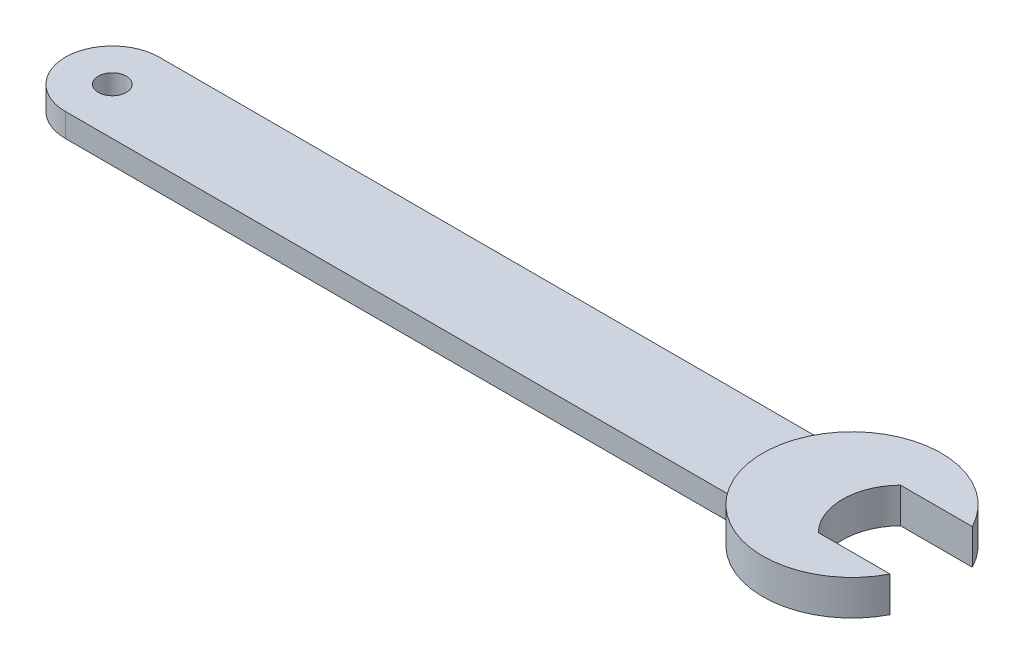
ISO-10303-21;
HEADER;
FILE_DESCRIPTION(('STEP AP214'),'2;1');
FILE_NAME('part.step','',(''),(''),'','','');
FILE_SCHEMA(('AUTOMOTIVE_DESIGN { 1 0 10303 214 1 1 1 1 }'));
ENDSEC;
DATA;
#1=APPLICATION_CONTEXT('core data for automotive mechanical design processes');
#2=APPLICATION_PROTOCOL_DEFINITION('international standard','automotive_design',2000,#1);
#3=PRODUCT_CONTEXT('',#1,'mechanical');
#4=PRODUCT('Part','Part','',(#3));
#5=PRODUCT_RELATED_PRODUCT_CATEGORY('part','',(#4));
#6=PRODUCT_DEFINITION_FORMATION('','',#4);
#7=PRODUCT_DEFINITION_CONTEXT('part definition',#1,'design');
#8=PRODUCT_DEFINITION('design','',#6,#7);
#9=PRODUCT_DEFINITION_SHAPE('','',#8);
#10=(LENGTH_UNIT() NAMED_UNIT(*) SI_UNIT(.MILLI.,.METRE.));
#11=(NAMED_UNIT(*) PLANE_ANGLE_UNIT() SI_UNIT($,.RADIAN.));
#12=(NAMED_UNIT(*) SI_UNIT($,.STERADIAN.) SOLID_ANGLE_UNIT());
#13=UNCERTAINTY_MEASURE_WITH_UNIT(LENGTH_MEASURE(1.E-05),#10,'distance_accuracy_value','');
#14=(GEOMETRIC_REPRESENTATION_CONTEXT(3) GLOBAL_UNCERTAINTY_ASSIGNED_CONTEXT((#13)) GLOBAL_UNIT_ASSIGNED_CONTEXT((#10,
#11,#12)) REPRESENTATION_CONTEXT('',''));
#15=CARTESIAN_POINT('',(0.,0.,0.));
#16=DIRECTION('',(0.,0.,1.));
#17=DIRECTION('',(1.,0.,0.));
#18=AXIS2_PLACEMENT_3D('',#15,#16,#17);
#19=CARTESIAN_POINT('',(0.,5.,-20.));
#20=DIRECTION('',(0.,0.,-1.));
#21=DIRECTION('',(-1.,0.,0.));
#22=AXIS2_PLACEMENT_3D('',#19,#20,#21);
#23=PLANE('',#22);
#24=DIRECTION('',(1.,0.,0.));
#25=VECTOR('',#24,1.);
#26=CARTESIAN_POINT('',(0.,-5.,-20.));
#27=LINE('',#26,#25);
#28=CARTESIAN_POINT('',(-157.5,-5.,-20.));
#29=VERTEX_POINT('',#28);
#30=CARTESIAN_POINT('',(125.189011157193,-5.,-20.0000000000001));
#31=VERTEX_POINT('',#30);
#32=EDGE_CURVE('E100',#29,#31,#27,.T.);
#33=ORIENTED_EDGE('',*,*,#32,.F.);
#34=DIRECTION('',(0.,-1.,0.));
#35=VECTOR('',#34,1.);
#36=CARTESIAN_POINT('',(-157.5,5.,-20.));
#37=LINE('',#36,#35);
#38=CARTESIAN_POINT('',(-157.5,5.,-20.));
#39=VERTEX_POINT('',#38);
#40=EDGE_CURVE('E49',#39,#29,#37,.T.);
#41=ORIENTED_EDGE('',*,*,#40,.F.);
#42=DIRECTION('',(1.,0.,0.));
#43=VECTOR('',#42,1.);
#44=CARTESIAN_POINT('',(0.,5.,-20.));
#45=LINE('',#44,#43);
#46=CARTESIAN_POINT('',(125.189011157193,5.,-20.));
#47=VERTEX_POINT('',#46);
#48=EDGE_CURVE('E111',#39,#47,#45,.T.);
#49=ORIENTED_EDGE('',*,*,#48,.T.);
#50=DIRECTION('',(0.,-1.,0.));
#51=VECTOR('',#50,1.);
#52=CARTESIAN_POINT('',(125.189011157193,5.,-20.0000000000001));
#53=LINE('',#52,#51);
#54=EDGE_CURVE('E11',#47,#31,#53,.T.);
#55=ORIENTED_EDGE('',*,*,#54,.T.);
#56=EDGE_LOOP('',(#33,#41,#49,#55));
#57=FACE_BOUND('',#56,.T.);
#58=ADVANCED_FACE('F41',(#57),#23,.T.);
#59=CARTESIAN_POINT('',(-157.5,5.,0.));
#60=DIRECTION('',(0.,-1.,0.));
#61=DIRECTION('',(0.,0.,-1.));
#62=AXIS2_PLACEMENT_3D('',#59,#60,#61);
#63=CYLINDRICAL_SURFACE('',#62,20.);
#64=CARTESIAN_POINT('',(-157.5,-5.,0.));
#65=DIRECTION('',(0.,1.,0.));
#66=DIRECTION('',(0.,0.,1.));
#67=AXIS2_PLACEMENT_3D('',#64,#65,#66);
#68=CIRCLE('',#67,20.);
#69=CARTESIAN_POINT('',(-157.5,-5.,20.));
#70=VERTEX_POINT('',#69);
#71=EDGE_CURVE('E95',#29,#70,#68,.T.);
#72=ORIENTED_EDGE('',*,*,#71,.T.);
#73=DIRECTION('',(0.,-1.,0.));
#74=VECTOR('',#73,1.);
#75=CARTESIAN_POINT('',(-157.5,5.,20.));
#76=LINE('',#75,#74);
#77=CARTESIAN_POINT('',(-157.5,5.,20.));
#78=VERTEX_POINT('',#77);
#79=EDGE_CURVE('E88',#78,#70,#76,.T.);
#80=ORIENTED_EDGE('',*,*,#79,.F.);
#81=CARTESIAN_POINT('',(-157.5,5.,0.));
#82=DIRECTION('',(0.,1.,0.));
#83=DIRECTION('',(0.,0.,1.));
#84=AXIS2_PLACEMENT_3D('',#81,#82,#83);
#85=CIRCLE('',#84,20.);
#86=EDGE_CURVE('E109',#39,#78,#85,.T.);
#87=ORIENTED_EDGE('',*,*,#86,.F.);
#88=ORIENTED_EDGE('',*,*,#40,.T.);
#89=EDGE_LOOP('',(#72,#80,#87,#88));
#90=FACE_BOUND('',#89,.T.);
#91=ADVANCED_FACE('F108',(#90),#63,.T.);
#92=CARTESIAN_POINT('',(-157.5,5.,0.));
#93=DIRECTION('',(0.,-1.,0.));
#94=DIRECTION('',(0.,0.,-1.));
#95=AXIS2_PLACEMENT_3D('',#92,#93,#94);
#96=CYLINDRICAL_SURFACE('',#95,6.00000000000002);
#97=CARTESIAN_POINT('',(-157.5,5.,0.));
#98=DIRECTION('',(0.,1.,0.));
#99=DIRECTION('',(0.,0.,1.));
#100=AXIS2_PLACEMENT_3D('',#97,#98,#99);
#101=CIRCLE('',#100,6.00000000000002);
#102=CARTESIAN_POINT('',(-157.5,5.,6.00000000000002));
#103=VERTEX_POINT('',#102);
#104=EDGE_CURVE('E93',#103,#103,#101,.T.);
#105=ORIENTED_EDGE('',*,*,#104,.T.);
#106=EDGE_LOOP('',(#105));
#107=FACE_BOUND('',#106,.T.);
#108=CARTESIAN_POINT('',(-157.5,-5.,0.));
#109=DIRECTION('',(0.,1.,0.));
#110=DIRECTION('',(0.,0.,1.));
#111=AXIS2_PLACEMENT_3D('',#108,#109,#110);
#112=CIRCLE('',#111,6.00000000000002);
#113=CARTESIAN_POINT('',(-157.5,-5.,6.00000000000002));
#114=VERTEX_POINT('',#113);
#115=EDGE_CURVE('E98',#114,#114,#112,.T.);
#116=ORIENTED_EDGE('',*,*,#115,.F.);
#117=EDGE_LOOP('',(#116));
#118=FACE_BOUND('',#117,.T.);
#119=ADVANCED_FACE('F43',(#107,#118),#96,.F.);
#120=CARTESIAN_POINT('',(0.,5.,20.));
#121=DIRECTION('',(0.,0.,-1.));
#122=DIRECTION('',(-1.,0.,0.));
#123=AXIS2_PLACEMENT_3D('',#120,#121,#122);
#124=PLANE('',#123);
#125=DIRECTION('',(1.,0.,0.));
#126=VECTOR('',#125,1.);
#127=CARTESIAN_POINT('',(0.,-5.,20.));
#128=LINE('',#127,#126);
#129=CARTESIAN_POINT('',(125.189011157193,-5.,19.9999999999999));
#130=VERTEX_POINT('',#129);
#131=EDGE_CURVE('E71',#70,#130,#128,.T.);
#132=ORIENTED_EDGE('',*,*,#131,.T.);
#133=DIRECTION('',(0.,-1.,0.));
#134=VECTOR('',#133,1.);
#135=CARTESIAN_POINT('',(125.189011157193,5.,19.9999999999999));
#136=LINE('',#135,#134);
#137=CARTESIAN_POINT('',(125.189011157193,5.,20.));
#138=VERTEX_POINT('',#137);
#139=EDGE_CURVE('E79',#138,#130,#136,.T.);
#140=ORIENTED_EDGE('',*,*,#139,.F.);
#141=DIRECTION('',(1.,0.,0.));
#142=VECTOR('',#141,1.);
#143=CARTESIAN_POINT('',(0.,5.,20.));
#144=LINE('',#143,#142);
#145=EDGE_CURVE('E59',#78,#138,#144,.T.);
#146=ORIENTED_EDGE('',*,*,#145,.F.);
#147=ORIENTED_EDGE('',*,*,#79,.T.);
#148=EDGE_LOOP('',(#132,#140,#146,#147));
#149=FACE_BOUND('',#148,.T.);
#150=ADVANCED_FACE('F86',(#149),#124,.F.);
#151=CARTESIAN_POINT('',(0.,5.,0.));
#152=DIRECTION('',(0.,1.,0.));
#153=DIRECTION('',(0.,0.,1.));
#154=AXIS2_PLACEMENT_3D('',#151,#152,#153);
#155=PLANE('',#154);
#156=ORIENTED_EDGE('',*,*,#104,.F.);
#157=EDGE_LOOP('',(#156));
#158=FACE_BOUND('',#157,.T.);
#159=CARTESIAN_POINT('',(157.5,5.,0.));
#160=DIRECTION('',(0.,1.,0.));
#161=DIRECTION('',(0.,0.,1.));
#162=AXIS2_PLACEMENT_3D('',#159,#160,#161);
#163=CIRCLE('',#162,38.);
#164=EDGE_CURVE('E81',#47,#138,#163,.T.);
#165=ORIENTED_EDGE('',*,*,#164,.F.);
#166=ORIENTED_EDGE('',*,*,#48,.F.);
#167=ORIENTED_EDGE('',*,*,#86,.T.);
#168=ORIENTED_EDGE('',*,*,#145,.T.);
#169=EDGE_LOOP('',(#165,#166,#167,#168));
#170=FACE_BOUND('',#169,.T.);
#171=ADVANCED_FACE('F119',(#158,#170),#155,.T.);
#172=CARTESIAN_POINT('',(0.,-5.,0.));
#173=DIRECTION('',(0.,1.,0.));
#174=DIRECTION('',(0.,0.,1.));
#175=AXIS2_PLACEMENT_3D('',#172,#173,#174);
#176=PLANE('',#175);
#177=ORIENTED_EDGE('',*,*,#115,.T.);
#178=EDGE_LOOP('',(#177));
#179=FACE_BOUND('',#178,.T.);
#180=CARTESIAN_POINT('',(157.5,-5.,0.));
#181=DIRECTION('',(0.,1.,0.));
#182=DIRECTION('',(0.,0.,1.));
#183=AXIS2_PLACEMENT_3D('',#180,#181,#182);
#184=CIRCLE('',#183,38.);
#185=EDGE_CURVE('E85',#31,#130,#184,.T.);
#186=ORIENTED_EDGE('',*,*,#185,.T.);
#187=ORIENTED_EDGE('',*,*,#131,.F.);
#188=ORIENTED_EDGE('',*,*,#71,.F.);
#189=ORIENTED_EDGE('',*,*,#32,.T.);
#190=EDGE_LOOP('',(#186,#187,#188,#189));
#191=FACE_BOUND('',#190,.T.);
#192=ADVANCED_FACE('F92',(#179,#191),#176,.F.);
#193=CARTESIAN_POINT('',(157.5,7.5,0.));
#194=DIRECTION('',(0.,-1.,0.));
#195=DIRECTION('',(0.,0.,-1.));
#196=AXIS2_PLACEMENT_3D('',#193,#194,#195);
#197=CYLINDRICAL_SURFACE('',#196,38.);
#198=CARTESIAN_POINT('',(157.5,-7.5,0.));
#199=DIRECTION('',(0.,1.,0.));
#200=DIRECTION('',(0.,0.,1.));
#201=AXIS2_PLACEMENT_3D('',#198,#199,#200);
#202=CIRCLE('',#201,38.);
#203=CARTESIAN_POINT('',(191.230549951046,-7.5,-17.5));
#204=VERTEX_POINT('',#203);
#205=CARTESIAN_POINT('',(191.230549951046,-7.5,17.5));
#206=VERTEX_POINT('',#205);
#207=EDGE_CURVE('E143',#204,#206,#202,.T.);
#208=ORIENTED_EDGE('',*,*,#207,.T.);
#209=DIRECTION('',(0.,-1.,0.));
#210=VECTOR('',#209,1.);
#211=CARTESIAN_POINT('',(191.230549951046,7.5,17.5));
#212=LINE('',#211,#210);
#213=CARTESIAN_POINT('',(191.230549951046,7.5,17.5));
#214=VERTEX_POINT('',#213);
#215=EDGE_CURVE('E128',#214,#206,#212,.T.);
#216=ORIENTED_EDGE('',*,*,#215,.F.);
#217=CARTESIAN_POINT('',(157.5,7.5,0.));
#218=DIRECTION('',(0.,1.,0.));
#219=DIRECTION('',(0.,0.,1.));
#220=AXIS2_PLACEMENT_3D('',#217,#218,#219);
#221=CIRCLE('',#220,38.);
#222=CARTESIAN_POINT('',(191.230549951046,7.5,-17.5));
#223=VERTEX_POINT('',#222);
#224=EDGE_CURVE('E155',#223,#214,#221,.T.);
#225=ORIENTED_EDGE('',*,*,#224,.F.);
#226=DIRECTION('',(0.,-1.,0.));
#227=VECTOR('',#226,1.);
#228=CARTESIAN_POINT('',(191.230549951046,7.5,-17.5));
#229=LINE('',#228,#227);
#230=EDGE_CURVE('E130',#223,#204,#229,.T.);
#231=ORIENTED_EDGE('',*,*,#230,.T.);
#232=EDGE_LOOP('',(#208,#216,#225,#231));
#233=FACE_BOUND('',#232,.T.);
#234=ORIENTED_EDGE('',*,*,#54,.F.);
#235=ORIENTED_EDGE('',*,*,#164,.T.);
#236=ORIENTED_EDGE('',*,*,#139,.T.);
#237=ORIENTED_EDGE('',*,*,#185,.F.);
#238=EDGE_LOOP('',(#234,#235,#236,#237));
#239=FACE_BOUND('',#238,.T.);
#240=ADVANCED_FACE('F78',(#233,#239),#197,.T.);
#241=CARTESIAN_POINT('',(178.5,7.5,0.));
#242=DIRECTION('',(0.,-1.,0.));
#243=DIRECTION('',(0.,0.,-1.));
#244=AXIS2_PLACEMENT_3D('',#241,#242,#243);
#245=CYLINDRICAL_SURFACE('',#244,25.);
#246=CARTESIAN_POINT('',(178.5,-7.5,0.));
#247=DIRECTION('',(0.,-1.,0.));
#248=DIRECTION('',(0.,0.,1.));
#249=AXIS2_PLACEMENT_3D('',#246,#247,#248);
#250=CIRCLE('',#249,25.);
#251=CARTESIAN_POINT('',(160.646428928643,-7.5,17.5));
#252=VERTEX_POINT('',#251);
#253=CARTESIAN_POINT('',(160.646428928643,-7.5,-17.5));
#254=VERTEX_POINT('',#253);
#255=EDGE_CURVE('E150',#252,#254,#250,.T.);
#256=ORIENTED_EDGE('',*,*,#255,.T.);
#257=DIRECTION('',(0.,-1.,0.));
#258=VECTOR('',#257,1.);
#259=CARTESIAN_POINT('',(160.646428928643,7.5,-17.5));
#260=LINE('',#259,#258);
#261=CARTESIAN_POINT('',(160.646428928643,7.5,-17.5));
#262=VERTEX_POINT('',#261);
#263=EDGE_CURVE('E105',#262,#254,#260,.T.);
#264=ORIENTED_EDGE('',*,*,#263,.F.);
#265=CARTESIAN_POINT('',(178.5,7.5,0.));
#266=DIRECTION('',(0.,-1.,0.));
#267=DIRECTION('',(0.,0.,1.));
#268=AXIS2_PLACEMENT_3D('',#265,#266,#267);
#269=CIRCLE('',#268,25.);
#270=CARTESIAN_POINT('',(160.646428928643,7.5,17.5));
#271=VERTEX_POINT('',#270);
#272=EDGE_CURVE('E136',#271,#262,#269,.T.);
#273=ORIENTED_EDGE('',*,*,#272,.F.);
#274=DIRECTION('',(0.,-1.,0.));
#275=VECTOR('',#274,1.);
#276=CARTESIAN_POINT('',(160.646428928643,7.5,17.5));
#277=LINE('',#276,#275);
#278=EDGE_CURVE('E134',#271,#252,#277,.T.);
#279=ORIENTED_EDGE('',*,*,#278,.T.);
#280=EDGE_LOOP('',(#256,#264,#273,#279));
#281=FACE_BOUND('',#280,.T.);
#282=ADVANCED_FACE('F175',(#281),#245,.F.);
#283=CARTESIAN_POINT('',(160.646428928643,7.5,-17.5));
#284=DIRECTION('',(0.,0.,-1.));
#285=DIRECTION('',(-1.,0.,0.));
#286=AXIS2_PLACEMENT_3D('',#283,#284,#285);
#287=PLANE('',#286);
#288=DIRECTION('',(1.,0.,0.));
#289=VECTOR('',#288,1.);
#290=CARTESIAN_POINT('',(160.646428928643,-7.5,-17.5));
#291=LINE('',#290,#289);
#292=EDGE_CURVE('E145',#254,#204,#291,.T.);
#293=ORIENTED_EDGE('',*,*,#292,.T.);
#294=ORIENTED_EDGE('',*,*,#230,.F.);
#295=DIRECTION('',(1.,0.,0.));
#296=VECTOR('',#295,1.);
#297=CARTESIAN_POINT('',(160.646428928643,7.5,-17.5));
#298=LINE('',#297,#296);
#299=EDGE_CURVE('E154',#262,#223,#298,.T.);
#300=ORIENTED_EDGE('',*,*,#299,.F.);
#301=ORIENTED_EDGE('',*,*,#263,.T.);
#302=EDGE_LOOP('',(#293,#294,#300,#301));
#303=FACE_BOUND('',#302,.T.);
#304=ADVANCED_FACE('F177',(#303),#287,.F.);
#305=CARTESIAN_POINT('',(160.646428928643,7.5,17.5));
#306=DIRECTION('',(0.,0.,1.));
#307=DIRECTION('',(1.,0.,0.));
#308=AXIS2_PLACEMENT_3D('',#305,#306,#307);
#309=PLANE('',#308);
#310=DIRECTION('',(-1.,0.,0.));
#311=VECTOR('',#310,1.);
#312=CARTESIAN_POINT('',(160.646428928643,-7.5,17.5));
#313=LINE('',#312,#311);
#314=EDGE_CURVE('E140',#206,#252,#313,.T.);
#315=ORIENTED_EDGE('',*,*,#314,.T.);
#316=ORIENTED_EDGE('',*,*,#278,.F.);
#317=DIRECTION('',(-1.,0.,0.));
#318=VECTOR('',#317,1.);
#319=CARTESIAN_POINT('',(160.646428928643,7.5,17.5));
#320=LINE('',#319,#318);
#321=EDGE_CURVE('E137',#214,#271,#320,.T.);
#322=ORIENTED_EDGE('',*,*,#321,.F.);
#323=ORIENTED_EDGE('',*,*,#215,.T.);
#324=EDGE_LOOP('',(#315,#316,#322,#323));
#325=FACE_BOUND('',#324,.T.);
#326=ADVANCED_FACE('F192',(#325),#309,.F.);
#327=CARTESIAN_POINT('',(178.5,7.5,0.));
#328=DIRECTION('',(0.,1.,0.));
#329=DIRECTION('',(0.,0.,1.));
#330=AXIS2_PLACEMENT_3D('',#327,#328,#329);
#331=PLANE('',#330);
#332=ORIENTED_EDGE('',*,*,#272,.T.);
#333=ORIENTED_EDGE('',*,*,#299,.T.);
#334=ORIENTED_EDGE('',*,*,#224,.T.);
#335=ORIENTED_EDGE('',*,*,#321,.T.);
#336=EDGE_LOOP('',(#332,#333,#334,#335));
#337=FACE_BOUND('',#336,.T.);
#338=ADVANCED_FACE('F162',(#337),#331,.T.);
#339=CARTESIAN_POINT('',(178.5,-7.5,0.));
#340=DIRECTION('',(0.,1.,0.));
#341=DIRECTION('',(0.,0.,1.));
#342=AXIS2_PLACEMENT_3D('',#339,#340,#341);
#343=PLANE('',#342);
#344=ORIENTED_EDGE('',*,*,#255,.F.);
#345=ORIENTED_EDGE('',*,*,#314,.F.);
#346=ORIENTED_EDGE('',*,*,#207,.F.);
#347=ORIENTED_EDGE('',*,*,#292,.F.);
#348=EDGE_LOOP('',(#344,#345,#346,#347));
#349=FACE_BOUND('',#348,.T.);
#350=ADVANCED_FACE('F193',(#349),#343,.F.);
#351=CLOSED_SHELL('',(#58,#91,#119,#150,#171,#192,#240,#282,#304,#326,#338,#350));
#352=MANIFOLD_SOLID_BREP('B2',#351);
#353=ADVANCED_BREP_SHAPE_REPRESENTATION('',(#18,#352),#14);
#354=SHAPE_DEFINITION_REPRESENTATION(#9,#353);
ENDSEC;
END-ISO-10303-21;
